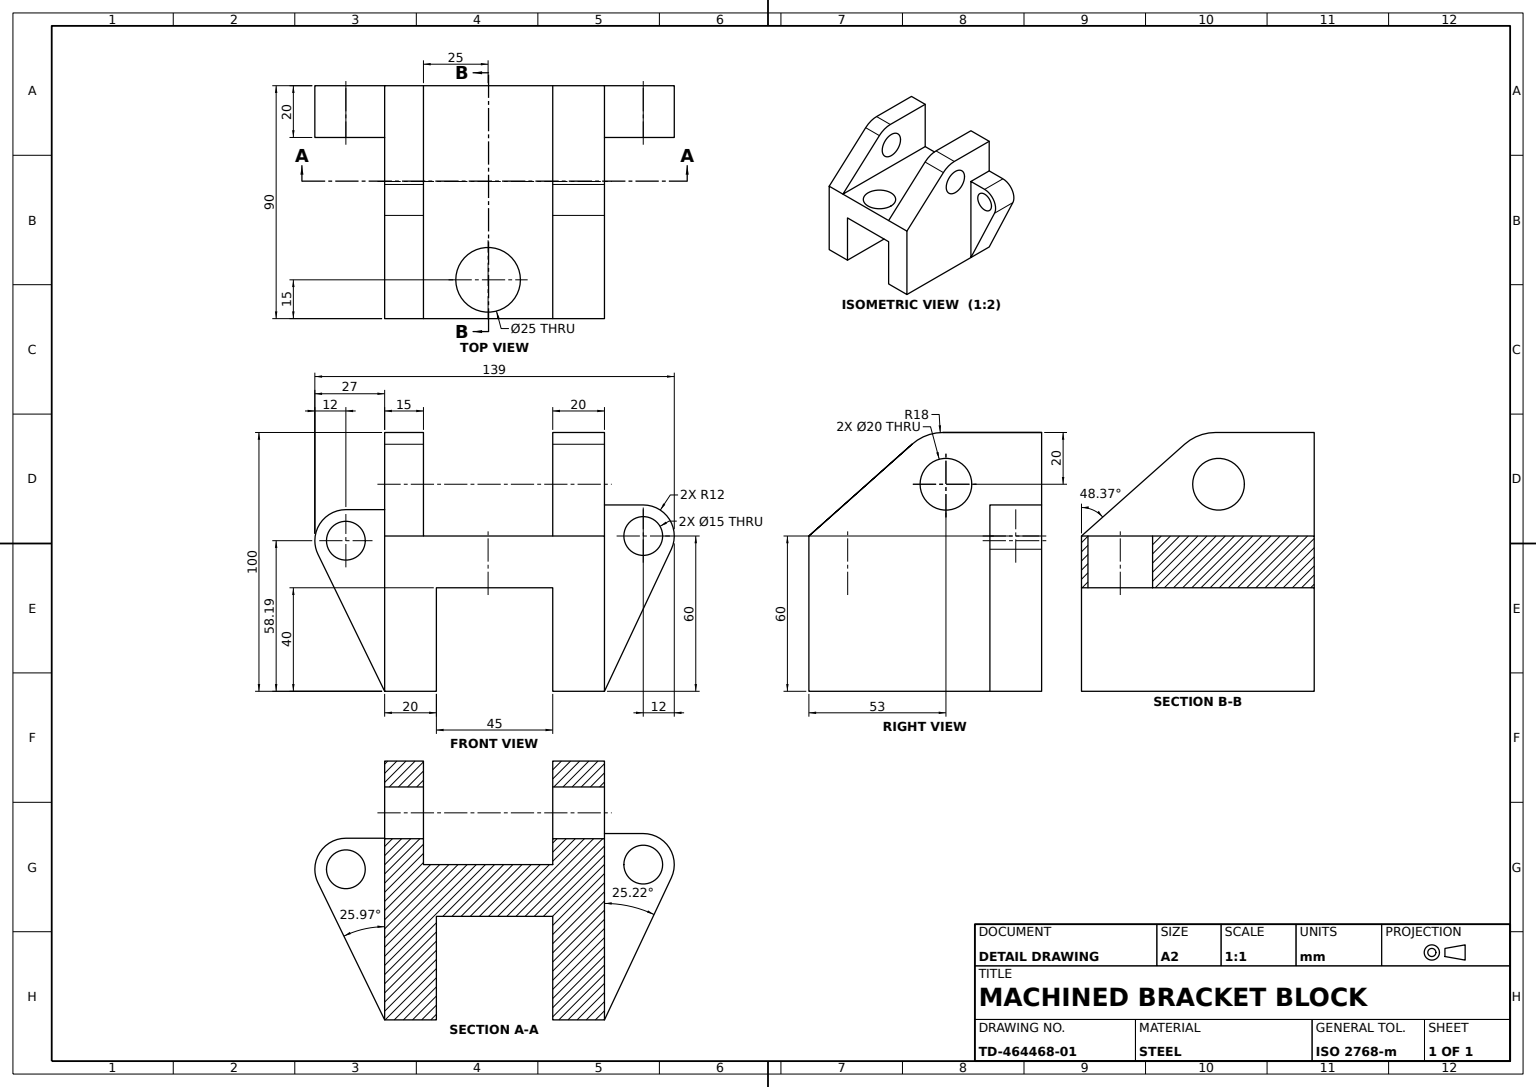
from build123d import *

# Parameters (mm, degrees)
BASE_BLOCK_SKETCH_W       = 90
BASE_BLOCK_SKETCH_H       = 45
BASE_BLOCK_90X45X60_DEPTH = 60
LUG_A_SKETCH_R            = 10
LUG_A_DEPTH               = 20
LUG_RECESS_CUT_DEPTH      = 5
LUG_B_DEPTH               = 20
LUG_HOLE_SKETCH_R         = 10
LUG_HOLES_DEPTH           = 114.357840488
ANGLED_SIDE_CUT_SKETCH_W  = 35
ANGLED_SIDE_CUT_SKETCH_H  = 40
ANGLED_SIDE_CUT_DEPTH     = 117.216392992
SIDE_BOSS_A_SKETCH_R      = 7.5
SIDE_BOSS_A_DEPTH         = 20
SIDE_BOSS_B_SKETCH_R      = 7.5
SIDE_BOSS_B_DEPTH         = 20
TOP_HOLE_SKETCH_R         = 12.5
TOP_HOLE_DEPTH            = 20
LUG_TOP_FILLET_R18_R      = 18
BOTTOM_SLOT_SKETCH_W      = 10
BOTTOM_SLOT_SKETCH_H      = 40
BOTTOM_SLOT_DEPTH         = 129.570019834


with BuildPart() as part:
    # Base Block Sketch → Base Block 90x45x60 (new body)
    with BuildSketch(Plane(origin=(0, 0, 0), x_dir=(1, 0, 0), z_dir=(0, 1, 0))):
        Rectangle(BASE_BLOCK_SKETCH_W, BASE_BLOCK_SKETCH_H)
    extrude(amount=-BASE_BLOCK_90X45X60_DEPTH)

    # Lug A Sketch → Lug A (add)
    with BuildSketch(Plane.XY.offset(22.5)):
        Polygon((-45, 0), (-45, -60), (45, -60), (45, 0), (0, 40), (-45, 40), align=None)
        with Locations((-8, 20)):
            Circle(LUG_A_SKETCH_R, mode=Mode.SUBTRACT)
    extrude(amount=LUG_A_DEPTH)

    # Lug Recess Sketch → Lug Recess Cut (cut)
    with BuildSketch(Plane(origin=(0, 0, 22.5), x_dir=(-1, 0, 0), z_dir=(0, 0, -1))):
        Polygon((-45, 0), (45, 0), (45, 40), (0, 40), align=None)
    extrude(amount=-LUG_RECESS_CUT_DEPTH, mode=Mode.SUBTRACT)

    # Lug B Sketch → Lug B (add)
    with BuildSketch(Plane(origin=(0, 0, -22.5), x_dir=(-1, 0, 0), z_dir=(0, 0, -1))):
        Polygon((-45, 0), (-45, -60), (45, -60), (45, 0), (45, 40), (0, 40), align=None)
    extrude(amount=LUG_B_DEPTH)

    # Lug Hole Sketch → Lug Holes (cut, through all)
    with BuildSketch(Plane.XY.offset(42.5)):
        with Locations((-8, 20)):
            Circle(LUG_HOLE_SKETCH_R)
    extrude(amount=-LUG_HOLES_DEPTH, mode=Mode.SUBTRACT)

    # Angled Side Cut Sketch → Angled Side Cut (cut, through all)
    with BuildSketch(Plane(origin=(45, 0, 0), x_dir=(0, 0, -1), z_dir=(1, 0, 0))):
        with Locations((-5, -40)):
            Rectangle(ANGLED_SIDE_CUT_SKETCH_W, ANGLED_SIDE_CUT_SKETCH_H)
    extrude(amount=-ANGLED_SIDE_CUT_DEPTH, mode=Mode.SUBTRACT)

    # Side Boss A Sketch → Side Boss A (add)
    with BuildSketch(Plane.ZY.offset(45)):
        with BuildLine():
            ThreePointArc((68.287962614, -7.064659931), (67.675104993, 4.552186853), (57.5, 10.190800338))
            Line((57.5, 10.190800338), (42.5, 10.190800338))
            Line((42.5, 10.190800338), (42.5, -60))
            Line((42.5, -60), (68.287962614, -7.064659931))
        make_face()
        with Locations((57.5, -1.809199662)):
            Circle(SIDE_BOSS_A_SKETCH_R, mode=Mode.SUBTRACT)
    extrude(amount=-SIDE_BOSS_A_DEPTH)

    # Side Boss B Sketch → Side Boss B (add)
    with BuildSketch(Plane.ZY.offset(45)):
        with BuildLine():
            Line((-42.5, 12), (-57.5, 12))
            ThreePointArc((-57.5, 12), (-67.633293922, 6.427779888), (-68.355763811, -5.113940953))
            Line((-68.355763811, -5.113940953), (-42.5, -60))
            Line((-42.5, -60), (-42.5, 12))
        make_face()
        with Locations((-57.5, 0)):
            Circle(SIDE_BOSS_B_SKETCH_R, mode=Mode.SUBTRACT)
    extrude(amount=-SIDE_BOSS_B_DEPTH)

    # Top Hole Sketch → Top Hole (cut)
    with BuildSketch(Plane(origin=(0, 0, 0), x_dir=(1, 0, 0), z_dir=(0, 1, 0))):
        with Locations(Location((30, -2.5, 0), (0, 0, 270))):
            Circle(TOP_HOLE_SKETCH_R)
    extrude(amount=-TOP_HOLE_DEPTH, mode=Mode.SUBTRACT)

    # Lug Top Fillet R18
    lug_top_fillet_r18_edges = [part.edges().sort_by_distance(p)[0] for p in [
        (0, 40, 35),
        (0, 40, -32.5),
    ]]
    fillet(lug_top_fillet_r18_edges, radius=LUG_TOP_FILLET_R18_R)

    # Bottom Slot Sketch → Bottom Slot (cut, through all)
    with BuildSketch(Plane(origin=(45, 0, 0), x_dir=(0, 0, -1), z_dir=(1, 0, 0))):
        with Locations((17.5, -40)):
            Rectangle(BOTTOM_SLOT_SKETCH_W, BOTTOM_SLOT_SKETCH_H)
    extrude(amount=-BOTTOM_SLOT_DEPTH, mode=Mode.SUBTRACT)


solid = part.part
